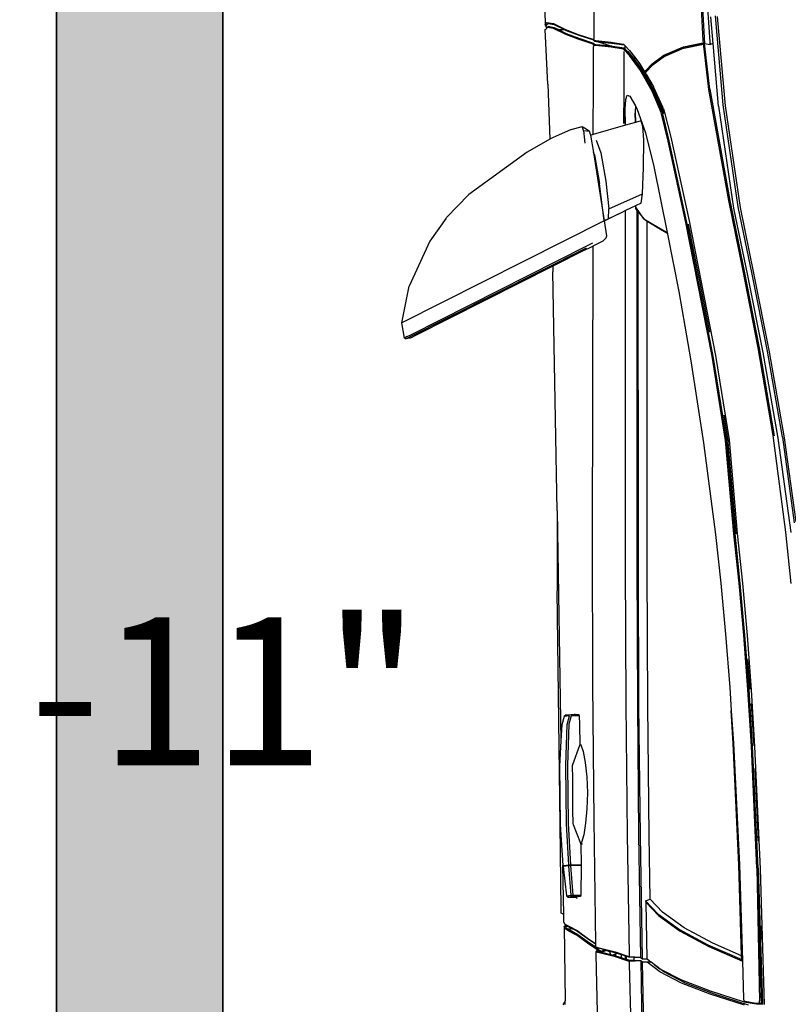
# Model space of a CAD drawing. Units: inches. Extents: x -4737294 to -4736756, y 1716389 to 1717040.
# Tile 8 of 25: x -4737217 to -4737176, y 1716543 to 1716597. Entities that reach past the tile are written whole.
import ezdxf

# ---------------------------------------------------------------- set-up
doc = ezdxf.new("R2010")
doc.units = ezdxf.units.IN
doc.header["$MEASUREMENT"] = 0
for name, color, linetype, lineweight in [('A-ANNO-DIMS', 2, 'Continuous', 18), ('A-EQPM-VEHI', 250, 'Continuous', 13), ('A-WALL-PATT', 244, 'Continuous', 13), ('walls', 252, 'Continuous', 35)]:
    doc.layers.add(name, color=color, linetype=linetype, lineweight=lineweight)
doc.layers.add('Edges', color=250, linetype='Continuous')
doc.styles.get("Standard").update_dxf_attribs({"font": 'arial.ttf'})
doc.dimstyles.get("Standard").update_dxf_attribs({"dimtxt": 8, "dimasz": 0.18, "dimexe": 0.18, "dimexo": 0.0625, "dimgap": 0.09, "dimtad": 0, "dimtih": 1, "dimtoh": 1, "dimzin": 0, "dimdsep": 46, "dimlunit": 3, "dimtxsty": 'Standard', "dimcen": 0.09, "dimadec": 0, "dimazin": 0, "dimtfac": 1, "dimtofl": 0, "dimtmove": 0, "dimatfit": 3, "dimfxl": 1, "dimtolj": 1, "dimtzin": 0, "dimarcsym": 0})

# ---------------------------------------------------------------- blocks, each defined once
blk = doc.blocks.new('Nissan Qashqai pl')
at = {"layer": 'Edges'}
for p, q in [((9.1605, 11.3208), (9.2669, 11.3354)), ((9.2656, 11.3376), (9.1612, 11.3233)), ((9.1617, 11.315), (9.2789, 11.331)), ((9.3422, 11.3316), (9.2783, 11.3251)), ((9.1605, 11.3208), (9.0538, 11.3023)), ((9.1612, 11.3233), (9.0546, 11.3048)), ((9.0552, 11.2965), (9.1617, 11.315)), ((9.2783, 11.3251), (9.1584, 11.3091)), ((9.0538, 11.3023), (8.9583, 11.2833)), ((9.0546, 11.3048), (8.9591, 11.2859)), ((9.1584, 11.3091), (9.0495, 11.2906)), ((9.0497, 11.2918), (9.1586, 11.3104)), ((9.0495, 11.2906), (8.9521, 11.2715)), ((8.9522, 11.2728), (9.0497, 11.2918)), ((8.9598, 11.2775), (9.0552, 11.2965)), ((9.6954, 11.2907), (9.5438, 11.2836)), ((9.5443, 11.2863), (9.696, 11.2932)), ((9.5717, 11.2865), (9.6618, 11.2907)), ((9.6953, 11.2892), (9.863, 11.2944)), ((9.6953, 11.2892), (9.8598, 11.2925)), ((9.6954, 11.2907), (9.8641, 11.2959)), ((9.696, 11.2932), (9.8644, 11.2982)), ((9.7669, 11.2945), (9.7832, 11.2951)), ((9.8629, 11.2925), (9.8598, 11.2925)), ((9.8626, 11.2878), (9.8627, 11.2909)), ((9.8627, 11.2909), (9.8629, 11.2925)), ((9.8627, 11.2909), (9.8637, 11.291)), ((9.8629, 11.2925), (9.863, 11.2944)), ((9.8641, 11.2959), (9.863, 11.2944)), ((9.8635, 11.2886), (9.8637, 11.291)), ((9.8637, 11.291), (9.8638, 11.2934)), ((9.8637, 11.291), (9.8643, 11.291)), ((9.8638, 11.2934), (9.8641, 11.2959)), ((8.9583, 11.2833), (8.8745, 11.266)), ((8.9591, 11.2859), (8.8754, 11.2687)), ((8.8761, 11.2602), (8.9598, 11.2775)), ((9.4735, 11.2779), (9.4062, 11.2729)), ((9.4736, 11.2793), (9.4063, 11.2743)), ((9.4064, 11.277), (9.4739, 11.282)), ((9.4727, 11.2808), (9.4362, 11.278)), ((9.4727, 11.2808), (9.4732, 11.2808)), ((9.5437, 11.2822), (9.4735, 11.2779)), ((9.5438, 11.2836), (9.4736, 11.2793)), ((9.4739, 11.282), (9.5443, 11.2863)), ((9.491, 11.2819), (9.5434, 11.2852)), ((9.6953, 11.2892), (9.5437, 11.2822)), ((9.8652, 11.2788), (9.8516, 11.2363)), ((9.8605, 11.2746), (9.8626, 11.2878)), ((9.8615, 11.2754), (9.8635, 11.2886)), ((8.8745, 11.266), (8.7481, 11.2473)), ((8.8754, 11.2687), (8.7491, 11.2501)), ((8.8666, 11.2554), (8.9522, 11.2728)), ((8.9521, 11.2715), (8.8666, 11.2541)), ((9.2801, 11.2648), (9.3418, 11.2713)), ((9.3418, 11.2671), (9.2803, 11.2606)), ((9.3419, 11.2685), (9.2804, 11.262)), ((9.3418, 11.2713), (9.4064, 11.277)), ((9.4062, 11.2729), (9.3418, 11.2671)), ((9.4063, 11.2743), (9.3419, 11.2685)), ((9.5403, 11.26), (9.6913, 11.2674)), ((9.6912, 11.2667), (9.5404, 11.2598)), ((9.8039, 11.27), (9.6912, 11.2667)), ((9.6913, 11.2674), (9.8099, 11.2711)), ((9.8039, 11.27), (9.7884, 11.2343)), ((9.7905, 11.2283), (9.8087, 11.2702)), ((9.7925, 11.2294), (9.8107, 11.2711)), ((9.8087, 11.2702), (9.8039, 11.27)), ((9.8099, 11.2711), (9.8087, 11.2702)), ((9.8099, 11.2711), (9.8107, 11.2711)), ((9.8107, 11.2711), (9.8573, 11.2726)), ((9.8475, 11.2312), (9.8611, 11.2734)), ((9.8652, 11.2738), (9.8516, 11.2313)), ((9.8573, 11.2726), (9.8603, 11.2727)), ((9.8603, 11.2727), (9.8605, 11.2746)), ((9.8611, 11.2734), (9.8603, 11.2727)), ((9.8612, 11.2735), (9.8611, 11.2734)), ((9.8612, 11.2735), (9.8615, 11.2754)), ((8.7287, 11.2307), (8.8666, 11.2554)), ((8.8666, 11.2541), (8.7292, 11.2295)), ((8.7496, 11.2416), (8.8761, 11.2602)), ((9.0591, 11.2377), (9.1639, 11.2546)), ((9.133, 11.2481), (9.1647, 11.2532)), ((9.1639, 11.2546), (9.2801, 11.2648)), ((9.2803, 11.2606), (9.1644, 11.2503)), ((9.2804, 11.262), (9.1645, 11.2518)), ((9.1647, 11.2532), (9.1668, 11.2533)), ((9.2804, 11.2635), (9.1668, 11.2533)), ((9.4048, 11.2501), (9.471, 11.2554)), ((9.471, 11.2554), (9.4997, 11.2573)), ((9.4997, 11.2573), (9.5403, 11.26)), ((9.5404, 11.2598), (9.4997, 11.2573)), ((8.7481, 11.2473), (8.6375, 11.2376)), ((8.7491, 11.2501), (8.6386, 11.2404)), ((8.7496, 11.2416), (8.6721, 11.2348)), ((9.1644, 11.2503), (9.06, 11.2335)), ((9.1645, 11.2518), (9.0601, 11.235)), ((9.2814, 11.2377), (9.3416, 11.2442)), ((9.3416, 11.2442), (9.4048, 11.2501)), ((8.6699, 11.231), (8.622, 11.228)), ((8.6721, 11.2348), (8.6387, 11.2319)), ((8.6721, 11.2312), (8.6699, 11.231)), ((8.6721, 11.2348), (8.6733, 11.2313)), ((8.6721, 11.2312), (8.6721, 11.2318)), ((8.6721, 11.2241), (8.6733, 11.2313)), ((8.6733, 11.2313), (8.6721, 11.2312)), ((8.7287, 11.2307), (8.6721, 11.2241)), ((8.7292, 11.2295), (8.6753, 11.2232)), ((9.0601, 11.235), (8.8941, 11.2023)), ((8.9679, 11.2201), (9.0591, 11.2377)), ((9.06, 11.2335), (8.9696, 11.2157)), ((8.9708, 11.2185), (9.03, 11.2304)), ((9.1676, 11.2229), (9.2814, 11.2377)), ((9.7884, 11.2343), (9.7692, 11.1989)), ((9.7733, 11.194), (9.7925, 11.2294)), ((9.8338, 11.1956), (9.8475, 11.2312)), ((9.8516, 11.2363), (9.8378, 11.2007)), ((9.8516, 11.2313), (9.8378, 11.1957)), ((8.6683, 11.2226), (8.6197, 11.2201)), ((8.6203, 11.2213), (8.6721, 11.2241)), ((8.671, 11.2227), (8.6683, 11.2226)), ((8.6721, 11.2241), (8.671, 11.2227)), ((8.6716, 11.2199), (8.671, 11.2227)), ((8.6759, 11.1982), (8.6716, 11.2199)), ((8.6721, 11.2241), (8.6727, 11.2229)), ((8.6772, 11.1988), (8.6721, 11.2241)), ((8.6753, 11.2232), (8.6727, 11.2229)), ((8.6777, 11.1984), (8.6727, 11.2229)), ((8.8918, 11.205), (8.9679, 11.2201)), ((8.9318, 11.211), (8.9704, 11.2185)), ((8.9704, 11.2185), (8.9708, 11.2185)), ((9.0656, 11.207), (9.1676, 11.2229)), ((9.7713, 11.1929), (9.7905, 11.2283)), ((8.7881, 11.1821), (8.8918, 11.205)), ((8.9696, 11.2157), (8.8942, 11.2009)), ((8.8961, 11.204), (8.9318, 11.211)), ((8.9797, 11.1924), (9.0656, 11.207)), ((8.6864, 11.1736), (8.6759, 11.1982)), ((8.6875, 11.1744), (8.6772, 11.1988)), ((8.6777, 11.1984), (8.6883, 11.1737)), ((8.8941, 11.2023), (8.7925, 11.1802)), ((8.8942, 11.2009), (8.7931, 11.1789)), ((8.9087, 11.1783), (8.9797, 11.1924)), ((9.7692, 11.1989), (9.7499, 11.1721)), ((9.7519, 11.1661), (9.7713, 11.1929)), ((9.754, 11.1672), (9.7733, 11.194)), ((9.8201, 11.1685), (9.8338, 11.1956)), ((9.8378, 11.2007), (9.8241, 11.1736)), ((9.8378, 11.1957), (9.8241, 11.1686)), ((8.7575, 11.1744), (8.7881, 11.1821)), ((8.7925, 11.1802), (8.7591, 11.1723)), ((8.697, 11.1592), (8.6864, 11.1736)), ((8.6979, 11.1603), (8.6875, 11.1744)), ((8.6883, 11.1737), (8.6987, 11.1597)), ((8.7508, 11.1722), (8.7257, 11.1609)), ((8.7529, 11.17), (8.7302, 11.1602)), ((8.7574, 11.1704), (8.7312, 11.1591)), ((8.7346, 11.1636), (8.7577, 11.1732)), ((8.7346, 11.1636), (8.7491, 11.1703)), ((8.7491, 11.1703), (8.7576, 11.1743)), ((8.7508, 11.1722), (8.7491, 11.1703)), ((8.7532, 11.1733), (8.7508, 11.1722)), ((8.7529, 11.17), (8.7577, 11.1732)), ((8.757, 11.1718), (8.7529, 11.17)), ((8.7532, 11.1733), (8.7575, 11.1744)), ((8.7587, 11.1722), (8.757, 11.1718)), ((8.7931, 11.1789), (8.7574, 11.1704)), ((8.7575, 11.1744), (8.7576, 11.1743)), ((8.7576, 11.1743), (8.7582, 11.1734)), ((8.7577, 11.1732), (8.7582, 11.1734)), ((8.7582, 11.1734), (8.759, 11.1725)), ((8.759, 11.1725), (8.7587, 11.1722)), ((8.7591, 11.1723), (8.7587, 11.1722)), ((8.759, 11.1725), (8.7591, 11.1723)), ((8.8245, 11.1613), (8.9063, 11.1779)), ((8.8893, 11.1486), (8.9021, 11.1697)), ((8.9041, 11.1717), (8.8927, 11.1528)), ((8.9021, 11.1697), (8.9063, 11.1779)), ((8.9075, 11.1781), (8.9041, 11.1717)), ((8.9063, 11.1779), (8.9075, 11.1781)), ((8.9075, 11.1781), (8.9087, 11.1783)), ((9.7499, 11.1721), (9.7337, 11.1566)), ((9.8241, 11.1686), (9.8119, 11.1529)), ((9.8241, 11.1736), (9.8147, 11.1616)), ((9.8147, 11.1616), (9.8201, 11.1685)), ((8.7055, 11.1514), (8.697, 11.1592)), ((8.6987, 11.1596), (8.6979, 11.1603)), ((8.6987, 11.1597), (8.6988, 11.1596)), ((8.6987, 11.1596), (8.6988, 11.1596)), ((8.6996, 11.1588), (8.6987, 11.1596)), ((8.6988, 11.1596), (8.6996, 11.1588)), ((8.6996, 11.1588), (8.6996, 11.1588)), ((8.7062, 11.1527), (8.6996, 11.1588)), ((8.6996, 11.1588), (8.7062, 11.1527)), ((8.7302, 11.1602), (8.7032, 11.145)), ((8.7312, 11.1591), (8.7042, 11.144)), ((8.7075, 11.1487), (8.7346, 11.1636)), ((8.7108, 11.1523), (8.7257, 11.1609)), ((8.7108, 11.1523), (8.7248, 11.1605)), ((8.7248, 11.1605), (8.7257, 11.1609)), ((8.7828, 11.1508), (8.8245, 11.1613)), ((9.6552, 11.1554), (9.4936, 11.1538)), ((9.7337, 11.1566), (9.6552, 11.1554)), ((9.7357, 11.1507), (9.7337, 11.1566)), ((9.7357, 11.1507), (9.7519, 11.1661)), ((9.7378, 11.1517), (9.754, 11.1672)), ((9.8078, 11.1528), (9.8119, 11.1579)), ((9.8147, 11.1616), (9.8119, 11.1579)), ((9.8119, 11.1579), (9.8119, 11.1529)), ((9.8147, 11.1616), (9.8147, 11.1616)), ((8.7042, 11.144), (8.687, 11.131)), ((8.6884, 11.1371), (8.6973, 11.144)), ((8.6917, 11.1371), (8.7075, 11.1487)), ((8.7032, 11.145), (8.6927, 11.1371)), ((8.6973, 11.144), (8.698, 11.1446)), ((8.698, 11.1446), (8.6981, 11.1446)), ((8.7071, 11.15), (8.6981, 11.1446)), ((8.707, 11.15), (8.7055, 11.1514)), ((8.7067, 11.1522), (8.7062, 11.1527)), ((8.7083, 11.1508), (8.7067, 11.1522)), ((8.707, 11.15), (8.7083, 11.1508)), ((8.7071, 11.15), (8.707, 11.15)), ((8.707, 11.15), (8.707, 11.15)), ((8.7083, 11.1508), (8.7071, 11.15)), ((8.7083, 11.1507), (8.7102, 11.1519)), ((8.7083, 11.1508), (8.7083, 11.1507)), ((8.7102, 11.1519), (8.7108, 11.1523)), ((8.7524, 11.1401), (8.7828, 11.1508)), ((8.7748, 11.1475), (8.7678, 11.1453)), ((8.7678, 11.1453), (8.7698, 11.1385)), ((8.7916, 11.1488), (8.7748, 11.1475)), ((8.8259, 11.1483), (8.7916, 11.1488)), ((8.8585, 11.1473), (8.8259, 11.1483)), ((8.87, 11.1455), (8.8585, 11.1473)), ((8.8771, 11.1054), (8.8585, 11.1473)), ((8.87, 11.1455), (8.8734, 11.1385)), ((8.8893, 11.1486), (8.8751, 11.1387)), ((8.881, 11.1418), (8.8893, 11.1486)), ((8.8913, 11.1506), (8.8893, 11.1486)), ((8.8927, 11.1528), (8.8913, 11.1506)), ((9.3225, 11.1531), (8.8927, 11.1528)), ((9.4936, 11.1538), (9.3225, 11.1531)), ((9.6552, 11.1445), (9.4936, 11.1428)), ((9.654, 11.1423), (9.8061, 11.1447)), ((9.8078, 11.1471), (9.6552, 11.1445)), ((9.7357, 11.1507), (9.7378, 11.1517)), ((9.8078, 11.1528), (9.7378, 11.1517)), ((9.8061, 11.1447), (9.8051, 11.1309)), ((9.8058, 11.1369), (9.8061, 11.1447)), ((9.8061, 11.1447), (9.8078, 11.1471)), ((9.8078, 11.1471), (9.8078, 11.1528)), ((9.8101, 11.1449), (9.8098, 11.1369)), ((9.8101, 11.1449), (9.9411, 11.1475)), ((9.8119, 11.1472), (9.8101, 11.1449)), ((9.8101, 11.1449), (9.8112, 11.1311)), ((9.8119, 11.1529), (9.8119, 11.1472)), ((9.9393, 11.1497), (9.8119, 11.1472)), ((8.6805, 11.1309), (8.6746, 11.1253)), ((8.687, 11.131), (8.6788, 11.1237)), ((8.6805, 11.1309), (8.6884, 11.1371)), ((8.6859, 11.132), (8.6817, 11.1282)), ((8.6818, 11.1288), (8.6902, 11.136)), ((8.6927, 11.1371), (8.6859, 11.132)), ((8.6884, 11.1371), (8.6917, 11.1371)), ((8.6902, 11.136), (8.6917, 11.1371)), ((8.6923, 11.1371), (8.6927, 11.1371)), ((8.7361, 11.1283), (8.7373, 11.1314)), ((8.7373, 11.1314), (8.7492, 11.1383)), ((8.7492, 11.1383), (8.7524, 11.1401)), ((8.7492, 11.1383), (8.7572, 11.1379)), ((8.7572, 11.1379), (8.7698, 11.1383)), ((8.7698, 11.1385), (8.7583, 11.1382)), ((8.7698, 11.1385), (8.7698, 11.1383)), ((8.7698, 11.1383), (8.7733, 11.126)), ((8.8734, 11.1385), (8.8793, 11.1261)), ((8.8734, 11.1385), (8.8768, 11.1385)), ((8.8751, 11.1387), (8.8768, 11.1385)), ((8.8768, 11.1385), (8.879, 11.1402)), ((8.879, 11.1402), (8.881, 11.1418)), ((8.879, 11.1402), (9.3198, 11.1403)), ((9.3225, 11.1421), (8.881, 11.1418)), ((9.3198, 11.1403), (9.4922, 11.1409)), ((9.4936, 11.1428), (9.3225, 11.1421)), ((9.4922, 11.1409), (9.654, 11.1423)), ((9.802, 11.1309), (9.6538, 11.1284)), ((9.8051, 11.1309), (9.802, 11.1309)), ((9.8044, 11.129), (9.8051, 11.1309)), ((9.8055, 11.1298), (9.8058, 11.1369)), ((9.8098, 11.1369), (9.8058, 11.1369)), ((9.8098, 11.1369), (9.8096, 11.13)), ((9.8112, 11.1311), (9.8106, 11.1292)), ((9.8143, 11.1312), (9.8112, 11.1311)), ((9.9414, 11.1341), (9.8143, 11.1312)), ((8.6703, 11.1081), (8.6727, 11.1235)), ((8.6714, 11.1088), (8.6737, 11.1245)), ((8.6727, 11.1235), (8.6737, 11.1245)), ((8.6737, 11.1245), (8.6746, 11.1253)), ((8.6746, 11.1253), (8.6785, 11.1253)), ((8.6777, 11.1246), (8.6755, 11.1099)), ((8.6788, 11.1237), (8.6764, 11.1083)), ((8.6785, 11.1253), (8.6777, 11.1246)), ((8.6815, 11.128), (8.6785, 11.1253)), ((8.6815, 11.128), (8.6818, 11.1288)), ((8.6817, 11.1282), (8.6815, 11.128)), ((8.6817, 11.1282), (8.6818, 11.1288)), ((8.6818, 11.1238), (8.7026, 11.1238)), ((8.7026, 11.1238), (8.7026, 11.1239)), ((8.7026, 11.1238), (8.7072, 11.1239)), ((8.7072, 11.1239), (8.7072, 11.1239)), ((8.7072, 11.1239), (8.7273, 11.1239)), ((8.7273, 11.1239), (8.7273, 11.124)), ((8.7273, 11.1239), (8.7354, 11.124)), ((8.7354, 11.1241), (8.7354, 11.124)), ((8.7354, 11.124), (8.742, 11.124)), ((8.7415, 11.1265), (8.7361, 11.1283)), ((8.7534, 11.1257), (8.7415, 11.1265)), ((8.742, 11.1241), (8.742, 11.124)), ((8.742, 11.124), (8.742, 11.1241)), ((8.742, 11.124), (8.742, 11.124)), ((8.742, 11.124), (8.7426, 11.124)), ((8.7426, 11.1241), (8.7426, 11.124)), ((8.7426, 11.124), (8.7433, 11.124)), ((8.7433, 11.1241), (8.7433, 11.124)), ((8.7433, 11.124), (8.7711, 11.1241)), ((8.7711, 11.1241), (8.7516, 11.1241)), ((8.7718, 11.126), (8.7534, 11.1257)), ((8.7733, 11.126), (8.7718, 11.126)), ((8.7733, 11.126), (8.7849, 11.0859)), ((9.3194, 11.1262), (8.8793, 11.1261)), ((8.8793, 11.1261), (8.8815, 11.1214)), ((8.8815, 11.1214), (8.892, 11.0998)), ((8.8815, 11.1214), (8.8895, 11.1048)), ((9.4919, 11.1269), (9.3194, 11.1262)), ((9.6538, 11.1284), (9.4919, 11.1269)), ((9.7992, 11.1133), (9.8044, 11.129)), ((9.803, 11.1212), (9.8014, 11.1176)), ((9.8014, 11.1176), (9.8026, 11.1212)), ((9.8026, 11.1212), (9.8041, 11.1256)), ((9.803, 11.1212), (9.8026, 11.1212)), ((9.8067, 11.1213), (9.803, 11.1212)), ((9.8041, 11.1256), (9.8045, 11.1268)), ((9.8041, 11.1256), (9.8081, 11.1256)), ((9.8067, 11.1213), (9.8044, 11.1142)), ((9.8045, 11.1268), (9.8046, 11.1271)), ((9.8045, 11.1268), (9.8085, 11.1268)), ((9.8046, 11.1271), (9.8055, 11.1298)), ((9.8086, 11.1271), (9.8046, 11.1271)), ((9.8106, 11.1292), (9.8054, 11.1135)), ((9.8081, 11.1256), (9.8067, 11.1213)), ((9.8085, 11.1268), (9.8081, 11.1256)), ((9.8086, 11.1271), (9.8085, 11.1268)), ((9.8096, 11.13), (9.8086, 11.1271)), ((8.6684, 11.0892), (8.6703, 11.1081)), ((8.6697, 11.0922), (8.6714, 11.1088)), ((8.6698, 11.0925), (8.6755, 11.1099)), ((8.6754, 11.1089), (8.6735, 11.0898)), ((8.6764, 11.1082), (8.6744, 11.0891)), ((8.6755, 11.1099), (8.6754, 11.1089)), ((8.6764, 11.1082), (8.6764, 11.1083)), ((9.7937, 11.0918), (9.7992, 11.1133)), ((9.7978, 11.1044), (9.7987, 11.108)), ((9.7987, 11.108), (9.8002, 11.1141)), ((9.7992, 11.1065), (9.7987, 11.108)), ((9.7992, 11.1065), (9.7987, 11.1053)), ((9.8027, 11.1078), (9.7992, 11.1065)), ((9.8054, 11.1135), (9.7999, 11.0919)), ((9.8002, 11.1141), (9.8008, 11.1157)), ((9.8027, 11.1078), (9.8003, 11.0983)), ((9.8008, 11.1157), (9.8014, 11.1176)), ((9.8014, 11.1139), (9.8008, 11.1157)), ((9.8043, 11.1139), (9.8014, 11.1139)), ((9.8031, 11.1093), (9.8014, 11.1139)), ((9.8031, 11.1093), (9.8027, 11.1078)), ((9.8043, 11.1139), (9.8031, 11.1093)), ((9.8044, 11.1142), (9.8043, 11.1139)), ((8.7917, 11.0895), (8.8075, 11.0955)), ((8.807, 11.0862), (8.8918, 11.0997)), ((8.8075, 11.0955), (8.8429, 11.1016)), ((8.8429, 11.1016), (8.8771, 11.1054)), ((8.8918, 11.0997), (8.8455, 11.0936)), ((8.8895, 11.1048), (8.8771, 11.1054)), ((8.8908, 11.1021), (8.8895, 11.1048)), ((8.8906, 11.1024), (8.8895, 11.1048)), ((8.8906, 11.1024), (8.8911, 11.1013)), ((8.892, 11.0998), (8.8908, 11.1021)), ((8.8911, 11.1013), (8.8919, 11.0997)), ((8.8911, 11.1013), (8.8919, 11.0998)), ((8.8919, 11.0997), (8.8911, 11.1013)), ((8.8919, 11.0997), (8.8918, 11.0997)), ((8.8918, 11.0997), (9.0186, 10.8486)), ((8.892, 11.0998), (8.8919, 11.0998)), ((8.8919, 11.0998), (8.8919, 11.0997)), ((8.8919, 11.0997), (8.8919, 11.0997)), ((8.9106, 11.1029), (8.892, 11.0998)), ((8.892, 11.0998), (8.892, 11.0998)), ((8.9131, 11.102), (8.9106, 11.1029)), ((8.9171, 11.0978), (8.9131, 11.102)), ((8.9171, 11.0978), (8.917, 11.0974)), ((8.9171, 11.0978), (8.9233, 11.0855)), ((9.7964, 11.0988), (9.7943, 11.0907)), ((9.7992, 11.0966), (9.7963, 11.0918)), ((9.7964, 11.0988), (9.7973, 11.1023)), ((9.7964, 11.0988), (9.7992, 11.0966)), ((9.7964, 11.0917), (9.7996, 11.0966)), ((9.7973, 11.1023), (9.7977, 11.1042)), ((9.7977, 11.1033), (9.7973, 11.1023)), ((9.7973, 11.1023), (9.7977, 11.1011)), ((9.7987, 11.1053), (9.7977, 11.1033)), ((9.7977, 11.1042), (9.7978, 11.1044)), ((9.7977, 11.1042), (9.7977, 11.1033)), ((9.7977, 11.1011), (9.7977, 11.0998)), ((9.7977, 11.1011), (9.7985, 11.099)), ((9.7977, 11.0998), (9.7985, 11.099)), ((9.7987, 11.1053), (9.7978, 11.1044)), ((9.7985, 11.099), (9.7989, 11.098)), ((9.7998, 11.0964), (9.7988, 11.0925)), ((9.7989, 11.098), (9.7998, 11.0976)), ((9.7998, 11.0976), (9.7992, 11.0966)), ((9.8002, 11.098), (9.7996, 11.0966)), ((9.8001, 11.0974), (9.7996, 11.0966)), ((9.7996, 11.0966), (9.7998, 11.0964)), ((9.8003, 11.0983), (9.7998, 11.0976)), ((9.8001, 11.0974), (9.7998, 11.0964)), ((9.8002, 11.098), (9.8001, 11.0974)), ((9.8003, 11.0983), (9.8002, 11.098)), ((8.5326, 11.0874), (8.6675, 11.0866)), ((8.6606, 11.0674), (8.6667, 11.0857)), ((8.6616, 11.0683), (8.6675, 11.0862)), ((8.6718, 11.0868), (8.6657, 11.0684)), ((8.6667, 11.0857), (8.6675, 11.0862)), ((8.6728, 11.0858), (8.6667, 11.0675)), ((8.6674, 11.0864), (8.6675, 11.0865)), ((8.6675, 11.0865), (8.6675, 11.0866)), ((8.6676, 11.0866), (8.6675, 11.0866)), ((8.6675, 11.0862), (8.6679, 11.0864)), ((8.6676, 11.0864), (8.6677, 11.0866)), ((8.6677, 11.0866), (8.6676, 11.0866)), ((8.6682, 11.0866), (8.6677, 11.0866)), ((8.6679, 11.0864), (8.6682, 11.0866)), ((8.6682, 11.087), (8.6684, 11.0888)), ((8.6692, 11.0876), (8.6682, 11.0866)), ((8.6682, 11.087), (8.6692, 11.0876)), ((8.6682, 11.0866), (8.6682, 11.087)), ((8.6684, 11.0888), (8.6684, 11.0892)), ((8.6684, 11.0888), (8.6685, 11.089)), ((8.6692, 11.0876), (8.6697, 11.0922)), ((8.6697, 11.0922), (8.6698, 11.0925)), ((8.6729, 11.0874), (8.6718, 11.0868)), ((8.674, 11.0864), (8.6728, 11.0858)), ((8.6733, 11.0875), (8.6729, 11.0874)), ((8.6735, 11.0898), (8.6733, 11.0875)), ((8.6742, 11.0866), (8.674, 11.0864)), ((8.6744, 11.0891), (8.6742, 11.0866)), ((8.6744, 11.0866), (8.6742, 11.0866)), ((8.6742, 11.0858), (8.6743, 11.086)), ((8.6744, 11.0864), (8.6744, 11.0866)), ((8.6773, 11.0865), (8.6744, 11.0866)), ((8.6791, 11.0864), (8.677, 11.0864)), ((8.6791, 11.0865), (8.6773, 11.0865)), ((8.6791, 11.0865), (8.6791, 11.0864)), ((8.6878, 11.0864), (8.6791, 11.0865)), ((8.7205, 11.0863), (8.6791, 11.0864)), ((8.6878, 11.0864), (8.6791, 11.0864)), ((8.6878, 11.0865), (8.6878, 11.0864)), ((8.6911, 11.0864), (8.6878, 11.0864)), ((8.7205, 11.0863), (8.6911, 11.0864)), ((8.7849, 11.0859), (8.7205, 11.0863)), ((8.7849, 11.0827), (8.7807, 11.0812)), ((8.7849, 11.0859), (8.7856, 11.0834)), ((8.7849, 11.0827), (8.7858, 11.0828)), ((8.7858, 11.0828), (8.7856, 11.0834)), ((8.7858, 11.0828), (8.807, 11.0862)), ((8.8102, 11.0874), (8.807, 11.0862)), ((8.8102, 11.0874), (8.8455, 11.0936)), ((8.9232, 11.0779), (8.9194, 11.0854)), ((8.9233, 11.0855), (9.2886, 11.0848)), ((8.925, 11.0821), (8.9233, 11.0855)), ((8.928, 11.0762), (8.925, 11.0821)), ((9.2886, 11.0848), (9.4673, 11.0852)), ((9.4673, 11.0852), (9.6358, 11.0866)), ((9.6358, 11.0866), (9.7887, 11.0889)), ((9.7832, 11.0805), (9.7887, 11.0889)), ((9.7842, 11.0814), (9.7891, 11.0889)), ((9.7933, 11.0892), (9.7883, 11.0815)), ((9.7887, 11.0889), (9.7891, 11.0889)), ((9.7891, 11.0889), (9.79, 11.0889)), ((9.7965, 11.0915), (9.7894, 11.0806)), ((9.79, 11.0889), (9.7931, 11.089)), ((9.7931, 11.089), (9.7934, 11.0906)), ((9.7931, 11.089), (9.7933, 11.0892)), ((9.7933, 11.0892), (9.7941, 11.0901)), ((9.7934, 11.0906), (9.7937, 11.0918)), ((9.7934, 11.0906), (9.7938, 11.0904)), ((9.7941, 11.0901), (9.7943, 11.0907)), ((9.7955, 11.0925), (9.7943, 11.0907)), ((9.7963, 11.0918), (9.7955, 11.0925)), ((9.7963, 11.0918), (9.7963, 11.0918)), ((9.7964, 11.0917), (9.7963, 11.0918)), ((9.7964, 11.0917), (9.7964, 11.0917)), ((9.7967, 11.0915), (9.7964, 11.0917)), ((9.7965, 11.0915), (9.7967, 11.0915)), ((9.7983, 11.0901), (9.7965, 11.0915)), ((9.7967, 11.0915), (9.7986, 11.0916)), ((9.7977, 11.0907), (9.7967, 11.0915)), ((9.7982, 11.0902), (9.7977, 11.0907)), ((9.7986, 11.0916), (9.7982, 11.0902)), ((9.7983, 11.0901), (9.7982, 11.0902)), ((9.7986, 11.0898), (9.7983, 11.0901)), ((9.7988, 11.0925), (9.7986, 11.0916)), ((9.7986, 11.0898), (9.7993, 11.0891)), ((9.7999, 11.0919), (9.7993, 11.0891)), ((9.7993, 11.0891), (9.8024, 11.0892)), ((9.8024, 11.0892), (9.9426, 11.0923)), ((8.7751, 11.0723), (8.7779, 11.0773)), ((8.7798, 11.0739), (8.7751, 11.0723)), ((8.7785, 11.0587), (8.7751, 11.0723)), ((8.7779, 11.0773), (8.7807, 11.0812)), ((8.7798, 11.0739), (8.7807, 11.0812)), ((8.7798, 11.0739), (8.7954, 11.0758)), ((9.0333, 10.8597), (8.9232, 11.0779)), ((9.0386, 10.8534), (8.9254, 11.0778)), ((8.928, 11.0762), (8.9483, 11.0359)), ((9.5422, 11.0706), (9.5422, 11.0716)), ((9.5422, 11.0706), (9.5424, 11.0707)), ((9.5423, 11.0696), (9.5422, 11.0706)), ((9.5424, 11.0707), (9.5503, 11.0736)), ((9.5426, 11.0695), (9.5424, 11.0707)), ((9.5503, 11.0736), (9.5641, 11.076)), ((9.5641, 11.076), (9.5818, 11.0782)), ((9.5818, 11.0782), (9.6016, 11.0791)), ((9.6016, 11.0791), (9.6215, 11.0782)), ((9.6215, 11.0782), (9.6395, 11.0766)), ((9.6395, 11.0766), (9.654, 11.0744)), ((9.6645, 11.0705), (9.6413, 11.0616)), ((9.654, 11.0744), (9.6633, 11.0715)), ((9.6633, 11.0715), (9.6645, 11.0705)), ((9.6655, 11.0708), (9.6645, 11.0705)), ((9.6655, 11.0728), (9.6655, 11.0708)), ((9.6655, 11.0708), (9.6911, 11.0709)), ((9.6911, 11.0709), (9.692, 11.0709)), ((9.6911, 11.0645), (9.6911, 11.0709)), ((9.692, 11.0709), (9.692, 11.0645)), ((9.692, 11.0709), (9.7287, 11.0708)), ((9.7287, 11.0708), (9.7305, 11.0704)), ((9.7288, 11.0609), (9.7287, 11.0708)), ((9.7305, 11.0704), (9.7313, 11.0644)), ((9.7305, 11.0704), (9.7306, 11.0607)), ((9.7728, 11.066), (9.7832, 11.0805)), ((9.7738, 11.067), (9.7842, 11.0814)), ((9.7883, 11.0815), (9.7778, 11.0671)), ((9.7894, 11.0806), (9.7788, 11.0661)), ((8.6546, 11.0516), (8.6606, 11.0674)), ((8.6556, 11.0524), (8.6616, 11.0683)), ((8.6657, 11.0684), (8.6598, 11.0529)), ((8.6667, 11.0675), (8.6608, 11.0521)), ((8.7785, 11.0587), (8.7891, 11.0353)), ((9.5037, 11.0635), (9.5045, 11.0628)), ((9.5044, 11.0586), (9.5045, 11.0628)), ((9.5052, 11.0524), (9.5044, 11.0586)), ((9.5045, 11.0683), (9.5063, 11.0687)), ((9.5045, 11.0628), (9.5045, 11.0683)), ((9.5063, 11.0687), (9.5061, 11.0586)), ((9.5061, 11.0586), (9.5167, 11.0559)), ((9.5063, 11.0687), (9.5168, 11.0691)), ((9.5168, 11.0691), (9.5423, 11.0696)), ((9.5426, 11.0695), (9.5423, 11.0696)), ((9.5667, 11.0609), (9.5426, 11.0695)), ((9.5678, 11.0604), (9.5667, 11.0609)), ((9.5846, 11.0606), (9.5678, 11.0604)), ((9.6236, 11.0609), (9.5846, 11.0606)), ((9.64, 11.0611), (9.6236, 11.0609)), ((9.6413, 11.0616), (9.64, 11.0611)), ((9.64, 11.0549), (9.6912, 11.0577)), ((9.6912, 11.0631), (9.6911, 11.0645)), ((9.692, 11.0631), (9.6912, 11.0631)), ((9.6912, 11.0577), (9.6912, 11.0631)), ((9.6913, 11.0556), (9.6912, 11.0577)), ((9.692, 11.0645), (9.692, 11.0631)), ((9.692, 11.0631), (9.6921, 11.0578)), ((9.6921, 11.0578), (9.7288, 11.0609)), ((9.6922, 11.0556), (9.6921, 11.0578)), ((9.7288, 11.0588), (9.6922, 11.0556)), ((9.7288, 11.0588), (9.7288, 11.0609)), ((9.7288, 11.0609), (9.7306, 11.0607)), ((9.7306, 11.0607), (9.7288, 11.0588)), ((9.7296, 11.0527), (9.7288, 11.0588)), ((9.7306, 11.0607), (9.7314, 11.0547)), ((9.733, 11.066), (9.7313, 11.0644)), ((9.7314, 11.0547), (9.7313, 11.0644)), ((9.7674, 11.0557), (9.7728, 11.066)), ((9.7684, 11.0567), (9.7717, 11.0631)), ((9.7717, 11.0631), (9.7707, 11.0593)), ((9.7707, 11.0593), (9.7709, 11.0549)), ((9.7717, 11.0631), (9.7738, 11.067)), ((9.7778, 11.0671), (9.7724, 11.0568)), ((9.7788, 11.0661), (9.7734, 11.0558)), ((8.6472, 11.0366), (8.6546, 11.0516)), ((8.6482, 11.0375), (8.655, 11.0513)), ((8.6608, 11.0521), (8.6534, 11.0369)), ((8.6598, 11.0529), (8.655, 11.0432)), ((8.655, 11.0513), (8.6556, 11.0524)), ((8.655, 11.0513), (8.655, 11.0432)), ((9.2517, 11.0411), (9.5372, 11.0459)), ((9.5052, 11.0524), (9.5069, 11.0501)), ((9.5168, 11.0537), (9.5061, 11.0564)), ((9.5061, 11.0564), (9.5069, 11.0501)), ((9.5069, 11.0501), (9.5176, 11.0469)), ((9.5167, 11.0559), (9.5679, 11.0543)), ((9.5679, 11.0521), (9.5168, 11.0537)), ((9.5176, 11.0469), (9.5372, 11.0459)), ((9.5372, 11.0459), (9.5689, 11.0442)), ((9.5679, 11.0543), (9.64, 11.0549)), ((9.6401, 11.0528), (9.5679, 11.0521)), ((9.6913, 11.0556), (9.6401, 11.0528)), ((9.641, 11.045), (9.6921, 11.0485)), ((9.7466, 11.0464), (9.641, 11.045)), ((9.692, 11.0499), (9.6913, 11.0556)), ((9.6922, 11.0499), (9.692, 11.0499)), ((9.6921, 11.0485), (9.692, 11.0499)), ((9.6922, 11.0499), (9.6921, 11.0485)), ((9.7526, 11.0495), (9.6921, 11.0485)), ((9.6922, 11.0556), (9.693, 11.0486)), ((9.6922, 11.0556), (9.6922, 11.0499)), ((9.693, 11.0486), (9.7296, 11.0527)), ((9.7296, 11.0527), (9.7314, 11.0547)), ((9.7511, 11.0463), (9.7466, 11.0464)), ((9.7526, 11.0495), (9.7511, 11.0463)), ((9.7623, 11.0497), (9.7526, 11.0495)), ((9.7623, 11.0497), (9.7643, 11.0504)), ((9.7643, 11.0504), (9.7652, 11.0514)), ((9.7643, 11.0504), (9.7648, 11.0513)), ((9.7648, 11.0513), (9.7664, 11.054)), ((9.7648, 11.0513), (9.7648, 11.0513)), ((9.7652, 11.0514), (9.7665, 11.0535)), ((9.7664, 11.054), (9.7674, 11.0557)), ((9.7665, 11.0537), (9.7664, 11.054)), ((9.7665, 11.0535), (9.7676, 11.0553)), ((9.7667, 11.0508), (9.7665, 11.0535)), ((9.7676, 11.0511), (9.7667, 11.0508)), ((9.7677, 11.0498), (9.7667, 11.0508)), ((9.7673, 11.0545), (9.7676, 11.0553)), ((9.7673, 11.0543), (9.7673, 11.0545)), ((9.7676, 11.0511), (9.7673, 11.0543)), ((9.7676, 11.0553), (9.7684, 11.0567)), ((9.7676, 11.0555), (9.7678, 11.056)), ((9.769, 11.0516), (9.7676, 11.0511)), ((9.7677, 11.0498), (9.8598, 11.0514)), ((9.77, 11.0506), (9.7677, 11.0498)), ((9.7677, 11.0498), (9.7677, 11.0498)), ((9.7712, 11.055), (9.769, 11.0516)), ((9.7734, 11.0558), (9.77, 11.0506)), ((9.7709, 11.0549), (9.7712, 11.055)), ((9.7724, 11.0568), (9.7712, 11.055)), ((9.8598, 11.0514), (9.8614, 11.0504)), ((9.8643, 11.0514), (9.8598, 11.0514)), ((9.8614, 11.0504), (9.8647, 11.0485)), ((8.646, 11.0289), (8.6468, 11.0337)), ((8.6468, 11.0337), (8.6472, 11.0366)), ((8.647, 11.03), (8.6468, 11.0337)), ((8.647, 11.03), (8.6482, 11.0375)), ((8.6524, 11.0378), (8.651, 11.0302)), ((8.6534, 11.0369), (8.652, 11.0292)), ((8.655, 11.0432), (8.6524, 11.0378)), ((8.7891, 11.0353), (8.7908, 11.0322)), ((8.9483, 11.0359), (8.9552, 11.0361)), ((8.9483, 11.0359), (9.0343, 10.8656)), ((9.2517, 11.0411), (8.9552, 11.0361)), ((9.2517, 11.0411), (9.351, 11.0411)), ((9.641, 11.045), (9.351, 11.0411)), ((9.5689, 11.0442), (9.641, 11.045)), ((8.5838, 11.0251), (8.6489, 11.0263)), ((8.6489, 11.0263), (8.646, 11.0289)), ((8.6498, 11.0273), (8.647, 11.03)), ((8.6527, 11.0286), (8.6489, 11.0263)), ((8.6524, 11.0289), (8.6498, 11.0273)), ((8.651, 11.0302), (8.652, 11.0292)), ((8.652, 11.0292), (8.6524, 11.0289)), ((8.6524, 11.0289), (8.6527, 11.0286)), ((8.6527, 11.0286), (8.6537, 11.0275)), ((8.6547, 11.0265), (8.6537, 11.0275)), ((8.6537, 11.0275), (8.6537, 11.0275)), ((8.7222, 11.0298), (8.6547, 11.0265)), ((8.7222, 11.0298), (8.7908, 11.0322)), ((8.7908, 11.0322), (8.8066, 11.0041)), ((8.8066, 11.0041), (8.8591, 10.9315)), ((8.8591, 10.9315), (8.8879, 10.9041)), ((8.8885, 10.9037), (8.8879, 10.9041)), ((8.8885, 10.9037), (8.9173, 10.8831)), ((8.9173, 10.8831), (8.9731, 10.8577)), ((9.0343, 10.8656), (9.0347, 10.8648)), ((9.0347, 10.8648), (9.0362, 10.8619)), ((9.0186, 10.8486), (8.9731, 10.8577)), ((9.0374, 10.8517), (9.0186, 10.8486)), ((9.0356, 10.8553), (9.0333, 10.8597)), ((9.0356, 10.8553), (9.0374, 10.8517)), ((9.0362, 10.8619), (9.037, 10.8603)), ((9.0371, 10.8601), (9.037, 10.8603)), ((9.0371, 10.8601), (9.0376, 10.8591)), ((9.0376, 10.8591), (9.0371, 10.8595)), ((9.0386, 10.8534), (9.0374, 10.8517)), ((9.0376, 10.8591), (9.0386, 10.8534))]:
    blk.add_line(p, q, dxfattribs=at)
blk = doc.blocks.new('car')
blk.add_blockref('Nissan Qashqai pl', (-9.7433, -11.9151))
blk = doc.blocks.new('*D59')
at = {"layer": 'A-ANNO-DIMS', "color": 0, "lineweight": -2, "transparency": 16777216}
for p, q in [((-4737196.539, 1716655.661), (-4737225.279, 1716655.661)), ((-4737225.099, 1716655.481), (-4737225.099, 1716564.479)), ((-4737225.099, 1716465.024), (-4737225.099, 1716556.026)), ((-4737196.539, 1716464.844), (-4737225.279, 1716464.844))]:
    blk.add_line(p, q, dxfattribs=at)
at = {"layer": 'A-ANNO-DIMS', "color": 0, "transparency": 16777216}
for points in [[(-4737225.129, 1716655.481), (-4737225.069, 1716655.481), (-4737225.099, 1716655.661)], [(-4737225.129, 1716465.024), (-4737225.069, 1716465.024), (-4737225.099, 1716464.844)]]:
    blk.add_solid(points, dxfattribs=at)
at = {"layer": 'Defpoints', "color": 0, "transparency": 16777216}
for p in [(-4737196.476, 1716655.661), (-4737225.099, 1716464.844), (-4737196.476, 1716464.844)]:
    blk.add_point(p, dxfattribs=at)
at = {"layer": 'A-ANNO-DIMS', "color": 0, "transparency": 16777216, "insert": (-4737225.099, 1716560.253), "char_height": 8, "attachment_point": 5}
blk.add_mtext('\\A1;CAR 15\'-11"', dxfattribs=at)

msp = doc.modelspace()

# ---------------------------------------------------------------- hatches: boundary and pattern name
at = {"layer": 'A-WALL-PATT'}
h = msp.add_hatch(color=256, dxfattribs=at)
h.dxf.hatch_style = 1
h.paths.add_polyline_path([(-4737206.144, 1716844.565), (-4737110.144, 1716844.565), (-4737110.144, 1716823.907), (-4737105.644, 1716823.907), (-4737105.644, 1716844.565), (-4737098.44, 1716844.565), (-4737098.44, 1716849.065), (-4737206.144, 1716849.065), (-4737206.144, 1716993.065), (-4736864.144, 1716993.065), (-4736864.144, 1716849.065), (-4736963.275, 1716849.065), (-4736994.446, 1716849.065), (-4736997.144, 1716849.065), (-4736997.144, 1716844.565), (-4736864.144, 1716844.565), (-4736864.144, 1716668.565), (-4736934.391, 1716668.565), (-4736934.391, 1716664.065), (-4736864.144, 1716664.065), (-4736864.144, 1716462.065), (-4736855.144, 1716462.065), (-4736855.144, 1717002.065), (-4737215.144, 1717002.065), (-4737215.144, 1716462.065), (-4737206.144, 1716462.065), (-4737206.144, 1716659.065), (-4737062.144, 1716659.065), (-4737062.144, 1716647.493), (-4737057.644, 1716647.493), (-4737057.644, 1716796.565), (-4737071.812, 1716796.565), (-4737071.812, 1716792.065), (-4737070.805, 1716792.065), (-4737062.144, 1716792.065), (-4737062.144, 1716668.065), (-4737206.144, 1716668.065), (-4737206.144, 1716792.065), (-4737093.784, 1716792.065), (-4737093.784, 1716796.565), (-4737206.144, 1716796.565)])

# ---------------------------------------------------------------- linework, layer by layer
at = {"layer": 'walls'}
for p, q in [((-4737215.144, 1716462.065), (-4737215.144, 1717002.065)), ((-4737206.144, 1716462.065), (-4737206.144, 1716659.065))]:
    msp.add_line(p, q, dxfattribs=at)

# ---------------------------------------------------------------- block references
at = {"layer": 'A-EQPM-VEHI', "xscale": 43.56002006885659, "yscale": 43.56002006885659, "zscale": 43.56002006885659, "rotation": 270}
msp.add_blockref('car', (-4737150.017, 1716548.61), dxfattribs=at)

# ---------------------------------------------------------------- dimensions: what is measured, and where the dimension line sits
at = {"layer": 'A-ANNO-DIMS'}
dim = msp.add_linear_dim(base=(-4737225.099, 1716464.844), p1=(-4737196.476, 1716655.661), p2=(-4737196.476, 1716464.844), angle=270, text='CAR <>', dimstyle='Standard', override={"dimdec": 1, "dimlfac": 1, "dimrnd": 0, "dimzin": 1, "dimdsep": 46, "dimlunit": 4, "dimfrac": 2}, dxfattribs=at)
dim.commit()
dim.dimension.update_dxf_attribs({"geometry": '*D59', "text_midpoint": (-4737225.099, 1716560.253)})

doc.saveas('drawing.dxf')
